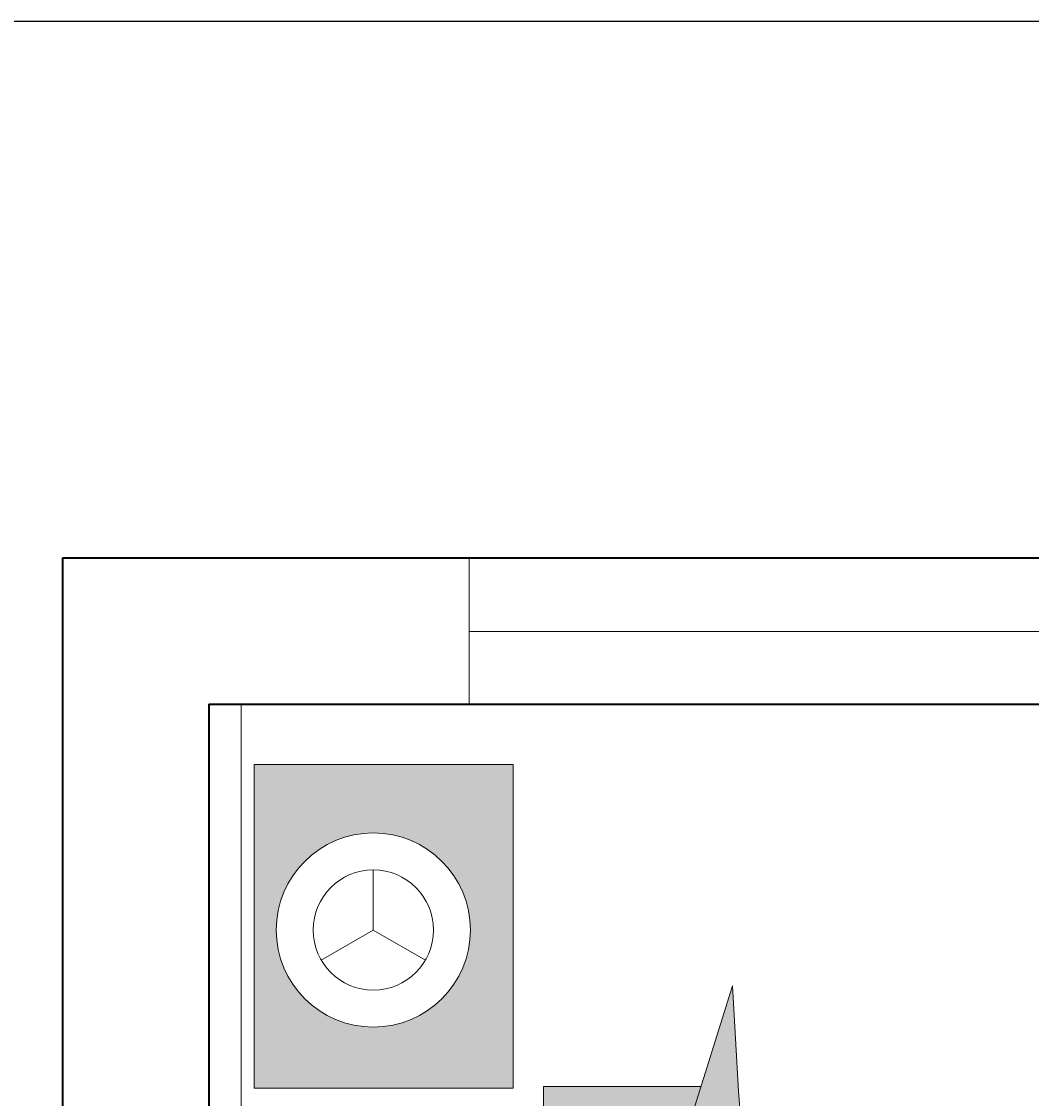
# Model space of a CAD drawing. Units: millimetres. Extents: x 27017497 to 27018854, y 7058029 to 7059154.
# Tile 45 of 91: x 27017611 to 27017673, y 7058557 to 7058623. Entities that reach past the tile are written whole.
import ezdxf

# ---------------------------------------------------------------- set-up
doc = ezdxf.new("R2010")
doc.units = ezdxf.units.MM
for name, color, linetype, lineweight in [('A-ANNO-DIMS', 2, 'Continuous', 18), ('A-FURN', 8, 'Continuous', 18), ('A-GLAZ', 4, 'Continuous', 18), ('A-WALL', 7, 'Continuous', 35)]:
    doc.layers.add(name, color=color, linetype=linetype, lineweight=lineweight)
doc.layers.add('A-FURN-PATT', color=177, linetype='Continuous', lineweight=13, true_color=0x293189)
doc.styles.get("Standard").update_dxf_attribs({"font": 'arial.ttf'})
doc.dimstyles.get("Standard").update_dxf_attribs({"dimtxt": 0.18, "dimasz": 0.18, "dimexe": 0.18, "dimexo": 0.0625, "dimgap": 0.09, "dimtad": 0, "dimtih": 1, "dimtoh": 1, "dimdec": 4, "dimzin": 0, "dimdsep": 46, "dimtxsty": 'Standard', "dimcen": 0.09, "dimadec": 0, "dimazin": 0, "dimtfac": 1, "dimtdec": 4, "dimtofl": 0, "dimtmove": 0, "dimatfit": 3, "dimfxl": 1, "dimtolj": 1, "dimtzin": 0, "dimarcsym": 0})

# ---------------------------------------------------------------- blocks, each defined once
blk = doc.blocks.new('CAMMAT')
for p, q in [((1.2731, 0), (-1.2731, 0)), ((1.2731, 0), (1.2731, -0.05)), ((1.2731, -0.05), (-1.2731, -0.05)), ((0.68, -0.07), (0.68, -0.47)), ((0.68, -0.07), (1.18, -0.07)), ((1.18, -0.07), (1.18, -0.47)), ((0.9242, -0.2541), (0.8777, -0.1737)), ((0.9242, -0.2541), (0.8777, -0.3346)), ((0.9242, -0.2541), (1.0171, -0.2541)), ((0.68, -0.47), (1.18, -0.47)), ((-0.6904, -0.5169), (0.6826, -0.5169)), ((0.6826, -0.5169), (0.6826, -0.7603)), ((0.0535, -0.5623), (0.8382, -0.8093))]:
    blk.add_line(p, q)
blk.add_lwpolyline([(0.8382, -0.8093), (0.6753, -0.8185), (0.5522, -0.828), (0.4622, -0.8406), (0.399, -0.8591), (0.356, -0.8862), (0.3267, -0.9248), (0.3046, -0.9777), (0.2832, -1.0476)])
for radius in [0.15, 0.0929]:
    blk.add_circle((0.9242, -0.2541), radius)
blk = doc.blocks.new('WINDOW-SINGLE-LIGHT')
blk.add_lwpolyline([(36, 4.5), (36, 0), (0, 0), (0, 9), (36, 9), (36, 4.5), (0, 4.5)])
blk = doc.blocks.new('*D48')
at = {"layer": 'A-ANNO-DIMS', "color": 0, "lineweight": -2, "transparency": 16777216}
for p, q in [((27018463.498, 7058622.912), (27017497.536, 7058622.912)), ((27017497.716, 7058622.732), (27017497.716, 7058357.753)), ((27017497.716, 7058092.41), (27017497.716, 7058357.389)), ((27018555.129, 7058092.23), (27017497.536, 7058092.23))]:
    blk.add_line(p, q, dxfattribs=at)
at = {"layer": 'A-ANNO-DIMS', "color": 0, "transparency": 16777216}
for points in [[(27017497.686, 7058622.732), (27017497.746, 7058622.732), (27017497.716, 7058622.912)], [(27017497.686, 7058092.41), (27017497.746, 7058092.41), (27017497.716, 7058092.23)]]:
    blk.add_solid(points, dxfattribs=at)
at = {"layer": 'Defpoints', "color": 0, "transparency": 16777216}
for p in [(27018463.561, 7058622.912), (27017497.716, 7058092.23), (27018555.192, 7058092.23)]:
    blk.add_point(p, dxfattribs=at)
at = {"layer": 'A-ANNO-DIMS', "color": 0, "transparency": 16777216, "insert": (27017497.716, 7058357.571), "char_height": 0.18, "attachment_point": 5}
blk.add_mtext('\\A1;530.7', dxfattribs=at)

msp = doc.modelspace()

# ---------------------------------------------------------------- hatches: boundary and pattern name
at = {"layer": 'A-FURN-PATT'}
h = msp.add_hatch(color=256, dxfattribs=at)
h.dxf.hatch_style = 1
h.paths.add_polyline_path([(27017701.132, 7058554.502, 0.414214), (27017699.539, 7058556.096), (27017655.346, 7058556.096), (27017655.646, 7058552.199), (27017656.148, 7058548.617), (27017656.883, 7058546.099), (27017657.965, 7058544.385), (27017659.503, 7058543.218), (27017661.609, 7058542.338), (27017664.394, 7058541.486), (27017661.59, 7058540.884), (27017659.349, 7058540.341), (27017657.446, 7058539.751), (27017655.654, 7058539.006), (27017653.746, 7058538), (27017651.496, 7058536.625), (27017648.677, 7058534.773), (27017645.063, 7058532.339), (27017648.677, 7058529.904), (27017651.496, 7058528.052), (27017653.746, 7058526.677), (27017655.654, 7058525.671), (27017657.446, 7058524.926), (27017659.349, 7058524.336), (27017661.59, 7058523.794), (27017664.394, 7058523.191), (27017661.609, 7058522.339), (27017659.503, 7058521.459), (27017657.965, 7058520.292), (27017656.883, 7058518.579), (27017656.148, 7058516.06), (27017655.646, 7058512.478), (27017655.268, 7058507.572), (27017655.084, 7058504.317), (27017699.539, 7058504.317, 0.414214), (27017701.132, 7058505.91)])
h.paths.add_polyline_path([(27017652.949, 7058557.393), (27017643.257, 7058557.393), (27017643.257, 7058502.708), (27017654.39, 7058502.708), (27017645.063, 7058532.339)])
h.paths.add_polyline_path([(27017656.883, 7058546.099), (27017656.148, 7058548.617), (27017655.646, 7058552.199), (27017655.268, 7058557.105), (27017654.901, 7058563.593), (27017645.063, 7058532.339), (27017648.677, 7058534.773), (27017651.496, 7058536.625), (27017653.746, 7058538), (27017655.654, 7058539.006), (27017657.446, 7058539.751), (27017659.349, 7058540.341), (27017661.59, 7058540.884), (27017664.394, 7058541.486), (27017661.609, 7058542.338), (27017659.503, 7058543.218), (27017657.965, 7058544.385)])
h.paths.add_polyline_path([(27017659.503, 7058521.459), (27017661.609, 7058522.339), (27017664.394, 7058523.191), (27017661.59, 7058523.794), (27017659.349, 7058524.336), (27017657.446, 7058524.926), (27017655.654, 7058525.671), (27017653.746, 7058526.677), (27017651.496, 7058528.052), (27017648.677, 7058529.904), (27017645.063, 7058532.339), (27017654.39, 7058502.708), (27017654.901, 7058501.084), (27017655.268, 7058507.572), (27017655.646, 7058512.478), (27017656.148, 7058516.06), (27017656.883, 7058518.579), (27017657.965, 7058520.292)])
h.paths.add_polyline_path([(27017640.173, 7058553.952, 0.414214), (27017638.978, 7058555.147), (27017629.419, 7058555.147, 0.414214), (27017628.224, 7058553.952), (27017628.224, 7058532.493, 0.414214), (27017629.419, 7058531.298), (27017638.978, 7058531.298, 0.414214), (27017640.173, 7058532.493)], flags=0)
h.paths.add_polyline_path([(27017640.173, 7058528.356, 0.414214), (27017638.978, 7058529.551), (27017629.419, 7058529.551, 0.414214), (27017628.224, 7058528.356), (27017628.224, 7058506.896, 0.414214), (27017629.419, 7058505.701), (27017638.978, 7058505.701, 0.414214), (27017640.173, 7058506.896)], flags=16)
h.paths.add_polyline_path([(27017643.257, 7058556.096), (27017627.049, 7058556.096, 0.414214), (27017625.455, 7058554.502), (27017625.455, 7058505.91, 0.414214), (27017627.049, 7058504.317), (27017643.257, 7058504.317)])
h.paths.add_polyline_path([(27017638.978, 7058531.298), (27017629.419, 7058531.298, -0.414214), (27017628.224, 7058532.493), (27017628.224, 7058553.952, -0.414214), (27017629.419, 7058555.147), (27017638.978, 7058555.147, -0.414214), (27017640.173, 7058553.952), (27017640.173, 7058532.493, -0.414214)], flags=16)
h.paths.add_polyline_path([(27017640.173, 7058528.356), (27017640.173, 7058506.896, -0.414214), (27017638.978, 7058505.701), (27017629.419, 7058505.701, -0.414214), (27017628.224, 7058506.896), (27017628.224, 7058528.356, -0.414214), (27017629.419, 7058529.551), (27017638.978, 7058529.551, -0.414214)], flags=0)
h.paths.add_polyline_path([(27017641.387, 7058503.122), (27017625.455, 7058503.122), (27017625.455, 7058483.207), (27017641.387, 7058483.207)])
h.paths.add_polyline_path([(27017626.814, 7058493.123, -1), (27017638.763, 7058493.123, -1)], flags=16)
h.paths.add_polyline_path([(27017629.088, 7058493.123, -1), (27017636.488, 7058493.123, -1)], flags=0)
h.paths.add_polyline_path([(27017641.387, 7058577.205), (27017625.455, 7058577.205), (27017625.455, 7058557.29), (27017641.387, 7058557.29)])
h.paths.add_polyline_path([(27017626.814, 7058567.015, -1), (27017638.763, 7058567.015, -1)], flags=16)
h.paths.add_polyline_path([(27017629.088, 7058567.015, -1), (27017636.488, 7058567.015, -1)], flags=0)

# ---------------------------------------------------------------- linework, layer by layer
at = {"layer": 'A-WALL'}
for p, q in [((27017613.666, 7058589.912), (27017613.666, 7058437.098)), ((27017613.666, 7058589.912), (27018310.606, 7058589.912)), ((27017622.666, 7058580.912), (27017622.666, 7058436.912)), ((27017622.666, 7058580.912), (27018223.606, 7058580.912))]:
    msp.add_line(p, q, dxfattribs=at)

# ---------------------------------------------------------------- block references
at = {"layer": 'A-FURN', "xscale": 39.82996475819422, "yscale": 39.82996475819422, "zscale": 39.82996475819422, "rotation": 89.99999999999999}
msp.add_blockref('CAMMAT', (27017622.667, 7058530.206), dxfattribs=at)
at = {"layer": 'A-GLAZ'}
msp.add_blockref('WINDOW-SINGLE-LIGHT', (27017638.686, 7058580.886), dxfattribs=at)

# ---------------------------------------------------------------- dimensions: what is measured, and where the dimension line sits
at = {"layer": 'A-ANNO-DIMS'}
dim = msp.add_linear_dim(base=(27017497.716, 7058092.23), p1=(27018463.561, 7058622.912), p2=(27018555.192, 7058092.23), angle=90, dimstyle='Standard', override={"dimdec": 1, "dimlfac": 1, "dimrnd": 0, "dimzin": 0, "dimdsep": 46, "dimlunit": 2}, dxfattribs=at)
dim.commit()
dim.dimension.update_dxf_attribs({"geometry": '*D48', "text_midpoint": (27017497.716, 7058357.571)})

doc.saveas('drawing.dxf')
